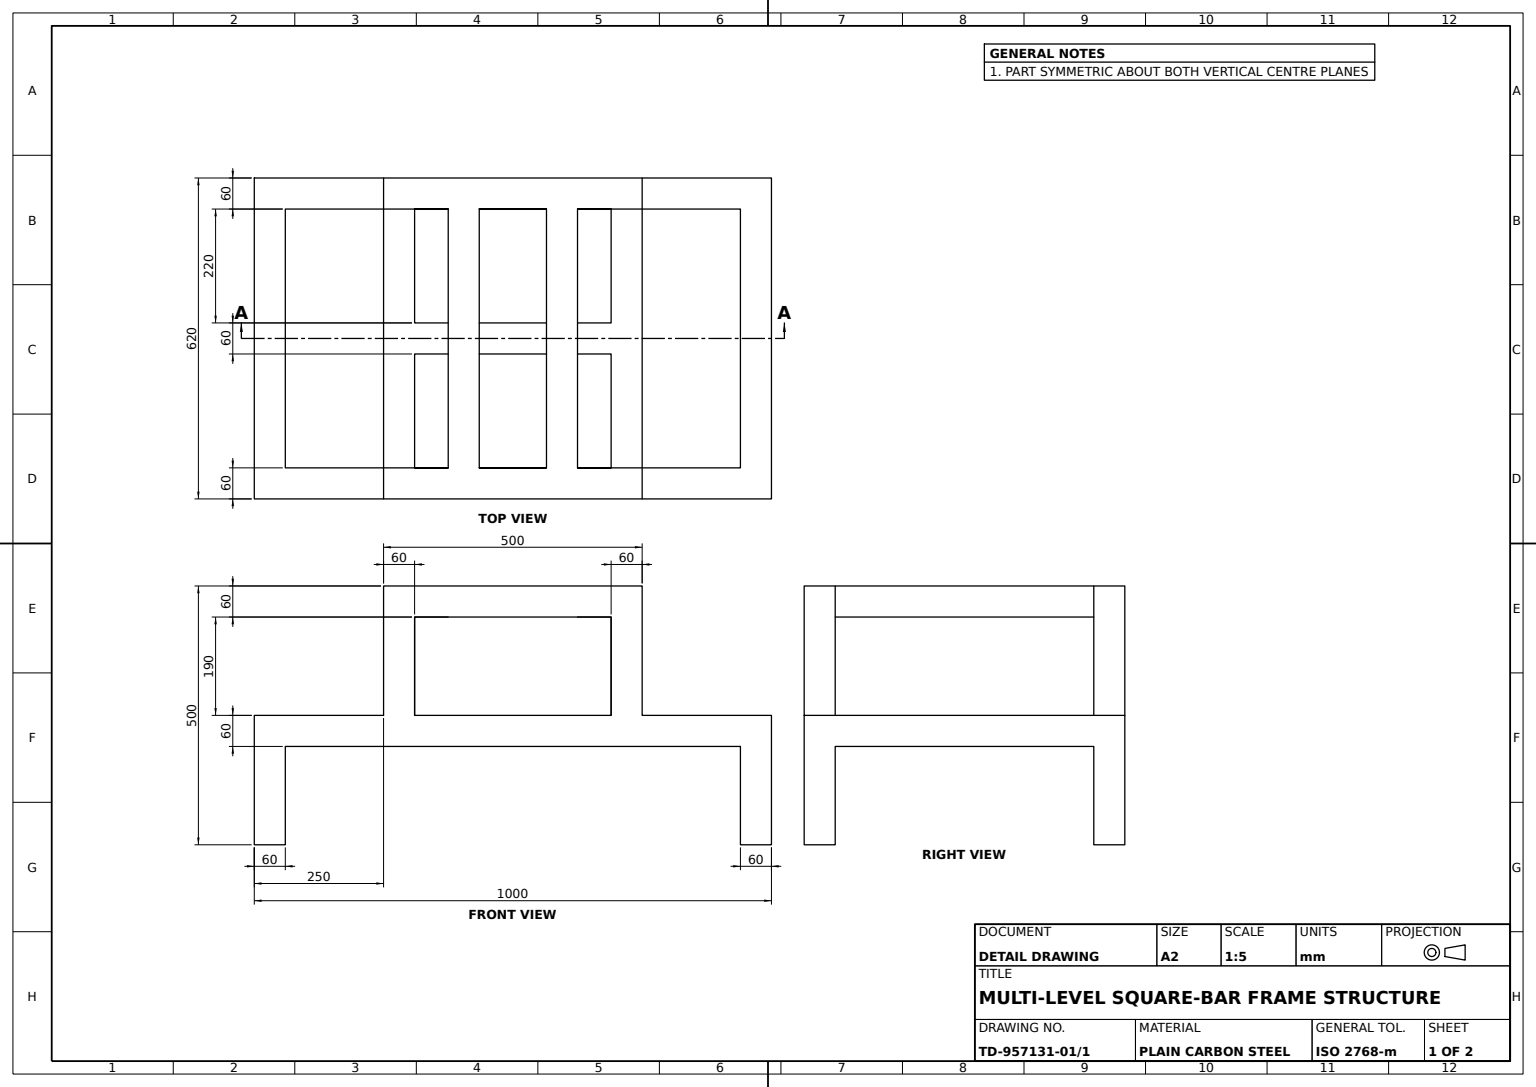
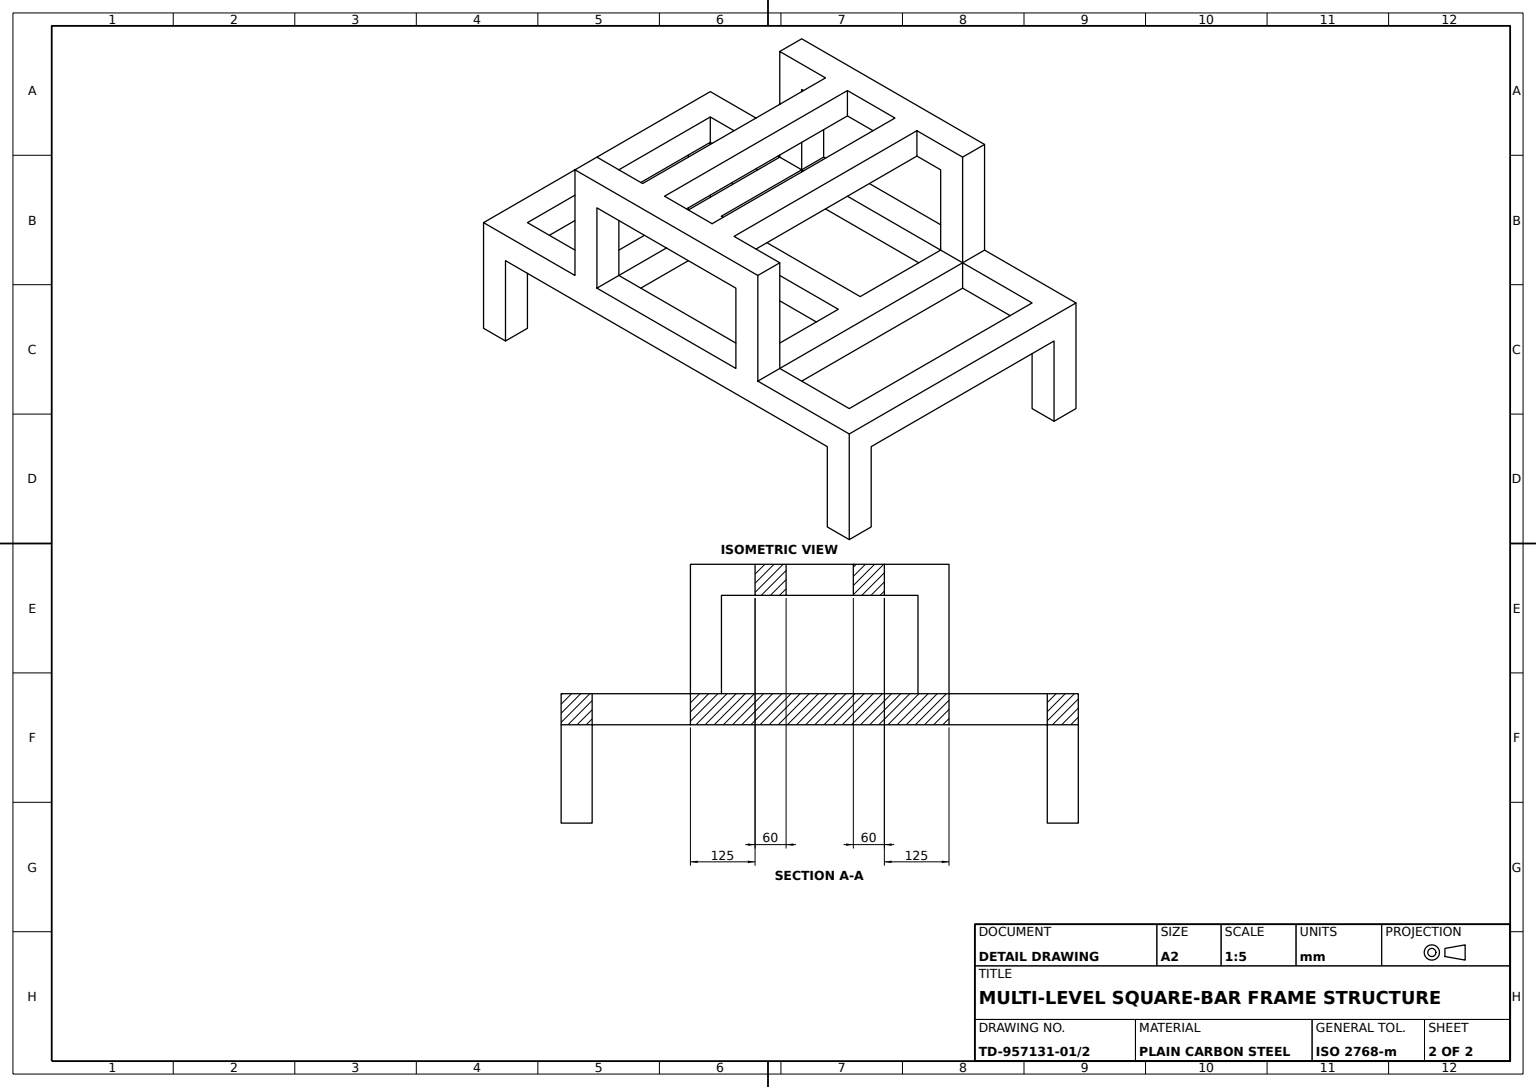
from build123d import *

# Parameters (mm, degrees)
FRONT_FRAME_DEPTH       = 60
FRAME_MEMBER_2_SKETCH_W = 60
FRAME_MEMBER_2_SKETCH_H = 500
FRAME_MEMBER_2_DEPTH    = 60
FRAME_MEMBER_3_DEPTH    = 60
FRAME_MEMBER_4_DEPTH    = 60
FRAME_MEMBER_5_DEPTH    = 60
FRAME_MEMBER_6_SKETCH_W = 60
FRAME_MEMBER_6_SKETCH_H = 500
FRAME_MEMBER_6_DEPTH    = 60
FRAME_MEMBER_7_DEPTH    = 60
FRAME_MEMBER_8_SKETCH_W = 60
FRAME_MEMBER_8_SKETCH_H = 500
FRAME_MEMBER_8_DEPTH    = 60


with BuildPart() as part:
    # Front Frame Sketch → Front Frame (new body)
    with BuildSketch(Plane.XY):
        Polygon((0, 0), (0, 250), (1000, 250), (1000, 0), (940, 0), (940, 190), (60, 190), (60, 0), align=None)
    extrude(amount=FRONT_FRAME_DEPTH)

    # Frame Member 2 Sketch → Frame Member 2 (add)
    with BuildSketch(Plane(origin=(0, 250, 0), x_dir=(1, 0, 0), z_dir=(0, 1, 0))):
        with Locations((30, 250)):
            Rectangle(FRAME_MEMBER_2_SKETCH_W, FRAME_MEMBER_2_SKETCH_H)
        with Locations((970, 250)):
            Rectangle(FRAME_MEMBER_2_SKETCH_W, FRAME_MEMBER_2_SKETCH_H)
    extrude(amount=-FRAME_MEMBER_2_DEPTH)

    # Frame Member 3 Sketch → Frame Member 3 (add)
    with BuildSketch(Plane(origin=(0, 0, -500), x_dir=(-1, 0, 0), z_dir=(0, 0, -1))):
        Polygon((-1000, 250), (0, 250), (0, 0), (-60, 0), (-60, 190), (-940, 190), (-940, 0), (-1000, 0), align=None)
    extrude(amount=FRAME_MEMBER_3_DEPTH)

    # Frame Member 4 Sketch → Frame Member 4 (add)
    with BuildSketch(Plane.XY.offset(60)):
        Polygon((750, 250), (750, 500), (250, 500), (250, 250), (310, 250), (310, 440), (690, 440), (690, 250), align=None)
    extrude(amount=-FRAME_MEMBER_4_DEPTH)

    # Frame Member 5 Sketch → Frame Member 5 (add)
    with BuildSketch(Plane(origin=(0, 0, -560), x_dir=(-1, 0, 0), z_dir=(0, 0, -1))):
        Polygon((-750, 250), (-750, 500), (-250, 500), (-250, 250), (-310, 250), (-310, 440), (-690, 440), (-690, 250), align=None)
    extrude(amount=-FRAME_MEMBER_5_DEPTH)

    # Frame Member 6 Sketch → Frame Member 6 (add)
    with BuildSketch(Plane(origin=(0, 250, 0), x_dir=(1, 0, 0), z_dir=(0, 1, 0))):
        with Locations((280, 250)):
            Rectangle(FRAME_MEMBER_6_SKETCH_W, FRAME_MEMBER_6_SKETCH_H)
        with Locations((720, 250)):
            Rectangle(FRAME_MEMBER_6_SKETCH_W, FRAME_MEMBER_6_SKETCH_H)
    extrude(amount=-FRAME_MEMBER_6_DEPTH)

    # Frame Member 7 Sketch → Frame Member 7 (add)
    with BuildSketch(Plane(origin=(0, 250, 0), x_dir=(1, 0, 0), z_dir=(0, 1, 0))):
        Polygon((310, 250), (310, 280), (690, 280), (690, 220), (310, 220), align=None)
    extrude(amount=-FRAME_MEMBER_7_DEPTH)

    # Frame Member 8 Sketch → Frame Member 8 (add)
    with BuildSketch(Plane(origin=(0, 500, 0), x_dir=(1, 0, 0), z_dir=(0, 1, 0))):
        with Locations((405, 250)):
            Rectangle(FRAME_MEMBER_8_SKETCH_W, FRAME_MEMBER_8_SKETCH_H)
        with Locations((595, 250)):
            Rectangle(FRAME_MEMBER_8_SKETCH_W, FRAME_MEMBER_8_SKETCH_H)
    extrude(amount=-FRAME_MEMBER_8_DEPTH)


solid = part.part
